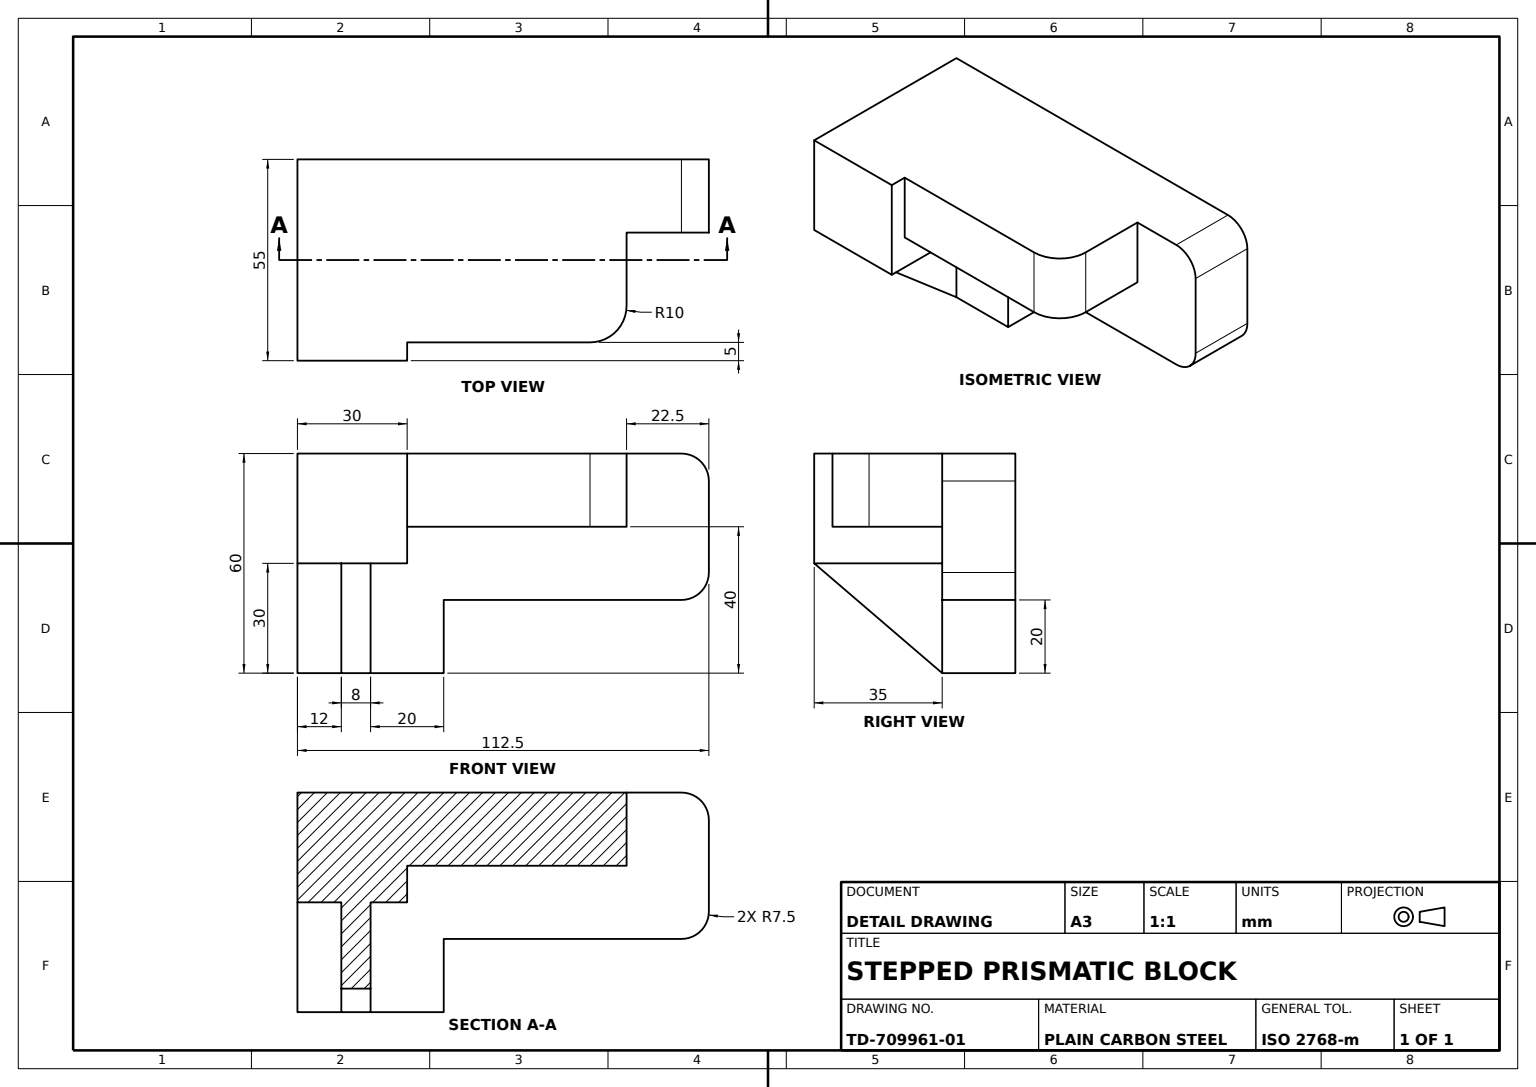
from build123d import *

# Parameters (mm, degrees)
BASE_BLOCK_DEPTH          = 20
SIDE_BLOCK_SKETCH_W       = 40
SIDE_BLOCK_SKETCH_H       = 20
SIDE_BLOCK_DEPTH          = 20
LONG_BLOCK_SKETCH_W       = 30
LONG_BLOCK_SKETCH_H       = 30
LONG_BLOCK_DEPTH          = 35
ROUNDED_END_BOSS_DEPTH    = 20
TRIANGULAR_GUSSET_DEPTH   = 20
TRIANGULAR_CUT_12MM_DEPTH = 12


with BuildPart() as part:
    # Base Block Sketch → Base Block (new body)
    with BuildSketch(Plane.XY):
        with BuildLine():
            Line((0, 0), (105, 0))
            ThreePointArc((105, 0), (110.303300859, 2.196699141), (112.5, 7.5))
            Line((112.5, 7.5), (112.5, 32.5))
            ThreePointArc((112.5, 32.5), (110.303300859, 37.803300859), (105, 40))
            Line((105, 40), (0, 40))
            Line((0, 40), (0, 0))
        make_face()
    extrude(amount=BASE_BLOCK_DEPTH)

    # Side Block Sketch → Side Block (add)
    with BuildSketch(Plane.XZ):
        with Locations((20, 10)):
            Rectangle(SIDE_BLOCK_SKETCH_W, SIDE_BLOCK_SKETCH_H)
    extrude(amount=SIDE_BLOCK_DEPTH)

    # Long Block Sketch → Long Block (add)
    with BuildSketch(Plane.XY.offset(20)):
        with Locations((15, 25)):
            Rectangle(LONG_BLOCK_SKETCH_W, LONG_BLOCK_SKETCH_H)
    extrude(amount=LONG_BLOCK_DEPTH)

    # Rounded End Sketch → Rounded End Boss (add)
    with BuildSketch(Plane(origin=(0, 40, 0), x_dir=(1, 0, 0), z_dir=(0, 1, 0))):
        with BuildLine():
            Line((80, -20), (30, -20))
            Line((30, -20), (30, -50))
            Line((30, -50), (80, -50))
            ThreePointArc((80, -50), (87.071067812, -47.071067812), (90, -40))
            Line((90, -40), (90, -20))
            Line((90, -20), (80, -20))
        make_face()
    extrude(amount=-ROUNDED_END_BOSS_DEPTH)

    # Triangular Gusset Sketch → Triangular Gusset (add)
    with BuildSketch(Plane.ZY):
        Polygon((20, 10), (55, 10), (20, -20), align=None)
    extrude(amount=-TRIANGULAR_GUSSET_DEPTH)

    # Triangular Cut Sketch → Triangular Cut 12mm (cut)
    with BuildSketch(Plane.ZY):
        Polygon((55, 10), (20, -20), (20, 10), align=None)
    extrude(amount=-TRIANGULAR_CUT_12MM_DEPTH, mode=Mode.SUBTRACT)


solid = part.part
